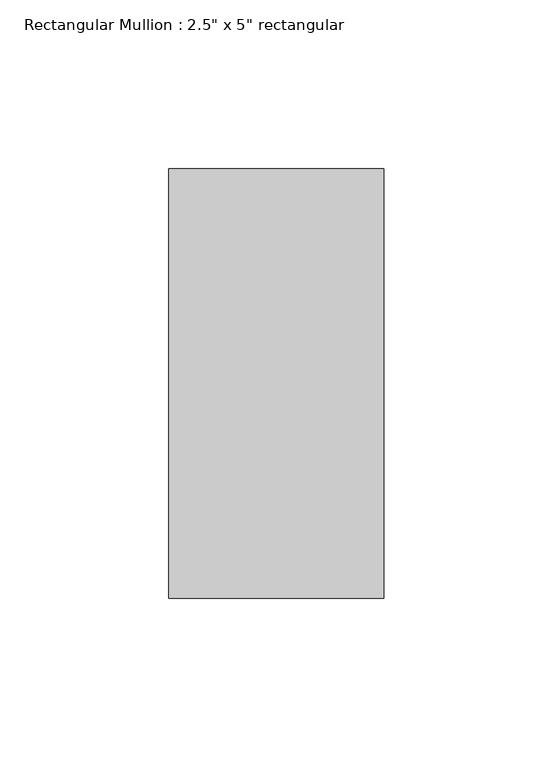
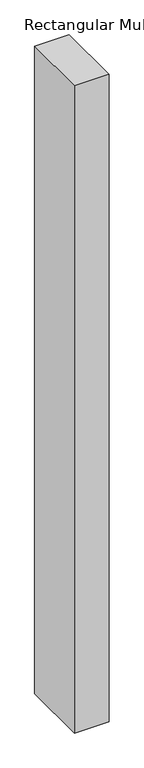
"""IFC4 building model written with IfcOpenShell, lengths in millimetres: member geometry."""

from ifc_helpers import new_model, si_unit, frame, origin, place, context, project, spatial, polyline, outline, extrude, source, transform, mapped, element, save


def member_16d8dc0e(model_context):
    return source(origin(), model_context, "Body", "SweptSolid", [
        extrude(outline(polyline([(0.0, 63.5), (0.0, -63.5), (-63.5, -63.5), (-63.5, 63.5), (0.0, 63.5)])), frame((0.0, 0.0, -1259.32546), z_axis=(0.0, 0.0, 1.0), x_axis=(1.0, 0.0, 0.0)), (0.0, 0.0, 1.0), 1259.32546),
    ])


if __name__ == "__main__":
    model = new_model("IFC4")
    model_context = context("Model", 3, world=origin())
    ifc_project = project(units=[si_unit("LENGTHUNIT", "METRE", prefix="MILLI")], contexts=[model_context])
    site = spatial("IfcSite", under=ifc_project)
    building = spatial("IfcBuilding", under=site)
    placement = place(None, origin())
    member_shape = member_16d8dc0e(model_context)
    element("IfcMember", 1, ObjectType="Rectangular Mullion : 2.5\" x 5\" rectangular", at=placement, inside=building, context=model_context, shape_type="MappedRepresentation", body=[
        mapped(member_shape, transform((0.0, 0.0, 0.0), x_axis=(1.0, 0.0, 0.0), y_axis=(0.0, 1.0, 0.0), z_axis=(0.0, 0.0, 1.0))),
    ])
    save(model, "model.ifc")

# Revit data of these elements
# Type "Rectangular Mullion : 2.5\" x 5\" rectangular"
#   built-in parameter 1007304 = 0.416667 (stored number, unit not read)
#   built-in parameter 1007301 = 0.104167 (stored number, unit not read)
#   built-in parameter 1007300 = 0.104167 (stored number, unit not read)
# Element 1 (IfcMember, "Rectangular Mullion : 2.5\" x 5\" rectangular")
#   Materials on its faces: "Iron, Ductile"
# Materials
#   "Iron, Ductile": class "Metal", colour RGB 0 0 0, transparency 0, Description = "Ductile cast iron", Cost = 0
